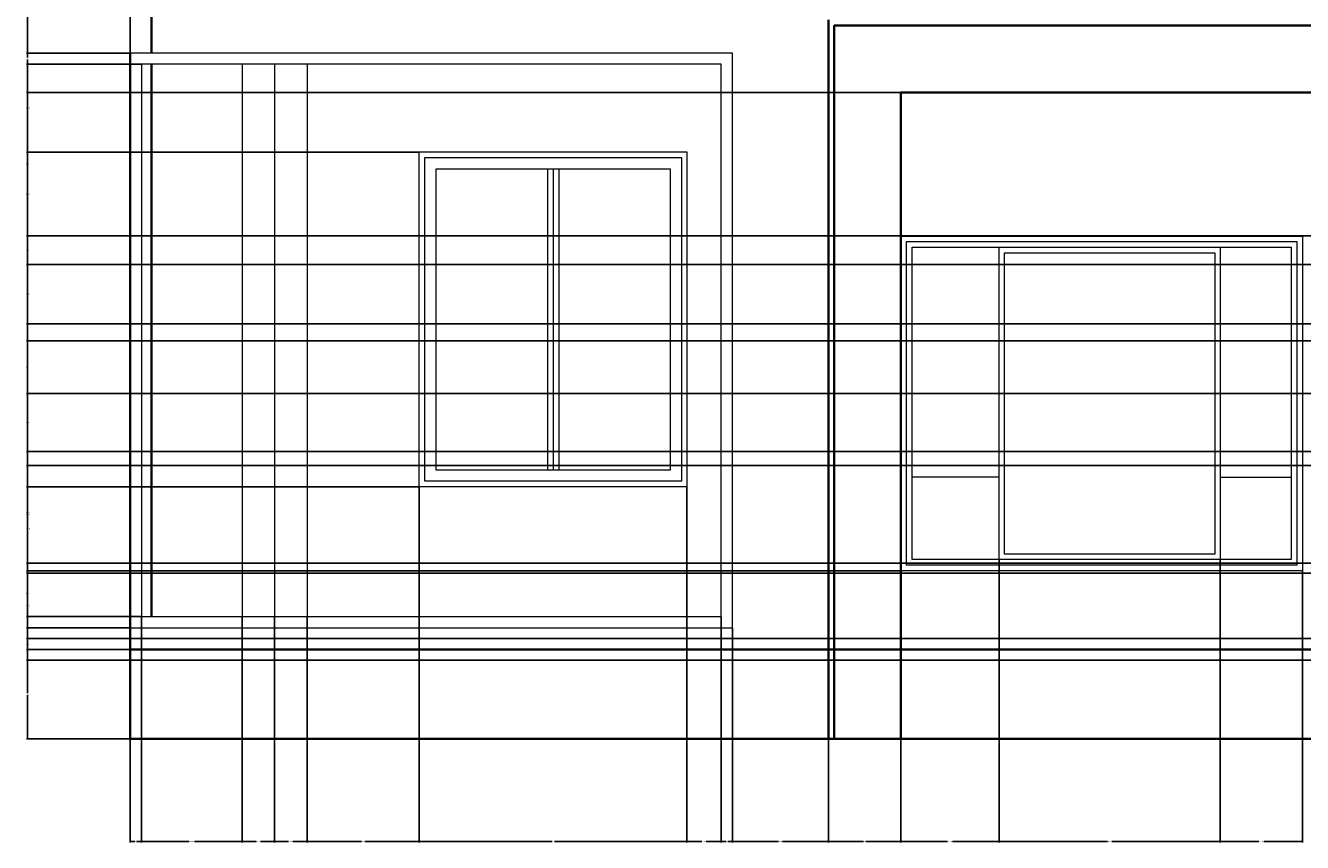
# Model space of a CAD drawing. Units: inches. Extents: x -7 to 391, y -12 to 303.
# Tile 1 of 5: x -7 to 222, y -12 to 134. Entities that reach past the tile are written whole.
import ezdxf

# ---------------------------------------------------------------- set-up
doc = ezdxf.new("R2010")
doc.units = ezdxf.units.IN
doc.header["$MEASUREMENT"] = 0
for name, color, linetype, lineweight in [('A-ANNO-DIMS', 2, 'Continuous', 18), ('A-DOOR', 3, 'Continuous', 18), ('A-ELEV', 7, 'Continuous', 35), ('A-GLAZ', 4, 'Continuous', 18)]:
    doc.layers.add(name, color=color, linetype=linetype, lineweight=lineweight)
doc.styles.get("Standard").update_dxf_attribs({"font": 'arial.ttf'})
doc.dimstyles.get("Standard").update_dxf_attribs({"dimtxt": 0.18, "dimasz": 0.18, "dimexe": 0.18, "dimexo": 0.0625, "dimgap": 0.09, "dimtad": 0, "dimtih": 1, "dimtoh": 1, "dimdec": 4, "dimzin": 0, "dimdsep": 46, "dimtxsty": 'Standard', "dimcen": 0.09, "dimadec": 0, "dimazin": 0, "dimtfac": 1, "dimtdec": 4, "dimtofl": 0, "dimtmove": 0, "dimatfit": 3, "dimfxl": 1, "dimtolj": 1, "dimtzin": 0, "dimarcsym": 0})

# ---------------------------------------------------------------- blocks, each defined once
blk = doc.blocks.new('*D1')
at = {"layer": 'A-ANNO-DIMS', "color": 0, "lineweight": -2, "transparency": 16777216}
for p, q in [((372.08, 122.18), (390.6, 122.18)), ((390.42, 122), (390.42, 64.44)), ((390.42, 6.53), (390.42, 64.08)), ((150.31, 6.35), (390.6, 6.35))]:
    blk.add_line(p, q, dxfattribs=at)
at = {"layer": 'A-ANNO-DIMS', "color": 0, "transparency": 16777216}
for points in [[(390.39, 122), (390.45, 122), (390.42, 122.18)], [(390.39, 6.53), (390.45, 6.53), (390.42, 6.35)]]:
    blk.add_solid(points, dxfattribs=at)
at = {"layer": 'Defpoints', "color": 0, "transparency": 16777216}
for p in [(372.02, 122.18), (390.42, 122.18), (150.24, 6.35)]:
    blk.add_point(p, dxfattribs=at)
at = {"layer": 'A-ANNO-DIMS', "color": 0, "transparency": 16777216, "insert": (390.42, 64.26), "char_height": 0.18, "attachment_point": 5}
blk.add_mtext('\\A1;115.83', dxfattribs=at)
blk = doc.blocks.new('*D7')
at = {"layer": 'A-ANNO-DIMS', "color": 0, "lineweight": -2, "transparency": 16777216}
for p, q in [((11.96, 22.35), (-6.56, 22.35)), ((-6.38, 22.17), (-6.38, 14.53)), ((-6.38, 6.53), (-6.38, 14.16)), ((11.96, 6.35), (-6.56, 6.35))]:
    blk.add_line(p, q, dxfattribs=at)
at = {"layer": 'A-ANNO-DIMS', "color": 0, "transparency": 16777216}
for points in [[(-6.41, 22.17), (-6.35, 22.17), (-6.38, 22.35)], [(-6.41, 6.53), (-6.35, 6.53), (-6.38, 6.35)]]:
    blk.add_solid(points, dxfattribs=at)
at = {"layer": 'Defpoints', "color": 0, "transparency": 16777216}
for p in [(-6.38, 22.35), (12.02, 22.35), (12.02, 6.35)]:
    blk.add_point(p, dxfattribs=at)
at = {"layer": 'A-ANNO-DIMS', "color": 0, "transparency": 16777216, "insert": (-6.38, 14.35), "char_height": 0.18, "attachment_point": 5}
blk.add_mtext('\\A1;16', dxfattribs=at)
blk = doc.blocks.new('*D8')
at = {"layer": 'A-ANNO-DIMS', "color": 0, "lineweight": -2, "transparency": 16777216}
for p, q in [((11.96, 26.25), (-6.56, 26.25)), ((-6.38, 26.07), (-6.38, 24.48)), ((-6.38, 22.53), (-6.38, 24.12)), ((11.96, 22.35), (-6.56, 22.35))]:
    blk.add_line(p, q, dxfattribs=at)
at = {"layer": 'A-ANNO-DIMS', "color": 0, "transparency": 16777216}
for points in [[(-6.41, 26.07), (-6.35, 26.07), (-6.38, 26.25)], [(-6.41, 22.53), (-6.35, 22.53), (-6.38, 22.35)]]:
    blk.add_solid(points, dxfattribs=at)
at = {"layer": 'Defpoints', "color": 0, "transparency": 16777216}
for p in [(-6.38, 26.25), (12.02, 26.25), (12.02, 22.35)]:
    blk.add_point(p, dxfattribs=at)
at = {"layer": 'A-ANNO-DIMS', "color": 0, "transparency": 16777216, "insert": (-6.38, 24.3), "char_height": 0.18, "attachment_point": 5}
blk.add_mtext('\\A1;3.905', dxfattribs=at)
blk = doc.blocks.new('*D9')
at = {"layer": 'A-ANNO-DIMS', "color": 0, "lineweight": -2, "transparency": 16777216}
for p, q in [((13.96, 28.25), (-6.56, 28.25)), ((-6.38, 28.07), (-6.38, 27.43)), ((11.96, 26.25), (-6.56, 26.25)), ((-6.38, 26.43), (-6.38, 27.07))]:
    blk.add_line(p, q, dxfattribs=at)
at = {"layer": 'A-ANNO-DIMS', "color": 0, "transparency": 16777216}
for points in [[(-6.41, 28.07), (-6.35, 28.07), (-6.38, 28.25)], [(-6.41, 26.43), (-6.35, 26.43), (-6.38, 26.25)]]:
    blk.add_solid(points, dxfattribs=at)
at = {"layer": 'Defpoints', "color": 0, "transparency": 16777216}
for p in [(-6.38, 28.25), (14.02, 28.25), (12.02, 26.25)]:
    blk.add_point(p, dxfattribs=at)
at = {"layer": 'A-ANNO-DIMS', "color": 0, "transparency": 16777216, "insert": (-6.38, 27.25), "char_height": 0.18, "attachment_point": 5}
blk.add_mtext('\\A1;2', dxfattribs=at)
blk = doc.blocks.new('*D10')
at = {"layer": 'A-ANNO-DIMS', "color": 0, "lineweight": -2, "transparency": 16777216}
for p, q in [((150.18, 36.46), (-6.56, 36.46)), ((-6.38, 36.28), (-6.38, 32.54)), ((-6.38, 28.43), (-6.38, 32.17)), ((13.96, 28.25), (-6.56, 28.25))]:
    blk.add_line(p, q, dxfattribs=at)
at = {"layer": 'A-ANNO-DIMS', "color": 0, "transparency": 16777216}
for points in [[(-6.41, 36.28), (-6.35, 36.28), (-6.38, 36.46)], [(-6.41, 28.43), (-6.35, 28.43), (-6.38, 28.25)]]:
    blk.add_solid(points, dxfattribs=at)
at = {"layer": 'Defpoints', "color": 0, "transparency": 16777216}
for p in [(-6.38, 36.46), (150.24, 36.46), (14.02, 28.25)]:
    blk.add_point(p, dxfattribs=at)
at = {"layer": 'A-ANNO-DIMS', "color": 0, "transparency": 16777216, "insert": (-6.38, 32.35), "char_height": 0.18, "attachment_point": 5}
blk.add_mtext('\\A1;8.206', dxfattribs=at)
blk = doc.blocks.new('*D11')
at = {"layer": 'A-ANNO-DIMS', "color": 0, "lineweight": -2, "transparency": 16777216}
for p, q in [((63.8, 51.51), (-6.56, 51.51)), ((-6.38, 51.33), (-6.38, 44.17)), ((-6.38, 36.64), (-6.38, 43.8)), ((150.18, 36.46), (-6.56, 36.46))]:
    blk.add_line(p, q, dxfattribs=at)
at = {"layer": 'A-ANNO-DIMS', "color": 0, "transparency": 16777216}
for points in [[(-6.41, 51.33), (-6.35, 51.33), (-6.38, 51.51)], [(-6.41, 36.64), (-6.35, 36.64), (-6.38, 36.46)]]:
    blk.add_solid(points, dxfattribs=at)
at = {"layer": 'Defpoints', "color": 0, "transparency": 16777216}
for p in [(-6.38, 51.51), (63.86, 51.51), (150.24, 36.46)]:
    blk.add_point(p, dxfattribs=at)
at = {"layer": 'A-ANNO-DIMS', "color": 0, "transparency": 16777216, "insert": (-6.38, 43.98), "char_height": 0.18, "attachment_point": 5}
blk.add_mtext('\\A1;15.058', dxfattribs=at)
blk = doc.blocks.new('*D12')
at = {"layer": 'A-ANNO-DIMS', "color": 0, "lineweight": -2, "transparency": 16777216}
for p, q in [((150.18, 96.46), (-6.56, 96.46)), ((-6.38, 96.28), (-6.38, 74.17)), ((-6.38, 51.69), (-6.38, 73.8)), ((63.8, 51.51), (-6.56, 51.51))]:
    blk.add_line(p, q, dxfattribs=at)
at = {"layer": 'A-ANNO-DIMS', "color": 0, "transparency": 16777216}
for points in [[(-6.41, 96.28), (-6.35, 96.28), (-6.38, 96.46)], [(-6.41, 51.69), (-6.35, 51.69), (-6.38, 51.51)]]:
    blk.add_solid(points, dxfattribs=at)
at = {"layer": 'Defpoints', "color": 0, "transparency": 16777216}
for p in [(-6.38, 96.46), (150.24, 96.46), (63.86, 51.51)]:
    blk.add_point(p, dxfattribs=at)
at = {"layer": 'A-ANNO-DIMS', "color": 0, "transparency": 16777216, "insert": (-6.38, 73.98), "char_height": 0.18, "attachment_point": 5}
blk.add_mtext('\\A1;44.94', dxfattribs=at)
blk = doc.blocks.new('*D13')
at = {"layer": 'A-ANNO-DIMS', "color": 0, "lineweight": -2, "transparency": 16777216}
for p, q in [((63.8, 111.51), (-6.56, 111.51)), ((-6.38, 111.33), (-6.38, 104.17)), ((-6.38, 96.64), (-6.38, 103.8)), ((150.18, 96.46), (-6.56, 96.46))]:
    blk.add_line(p, q, dxfattribs=at)
at = {"layer": 'A-ANNO-DIMS', "color": 0, "transparency": 16777216}
for points in [[(-6.41, 111.33), (-6.35, 111.33), (-6.38, 111.51)], [(-6.41, 96.64), (-6.35, 96.64), (-6.38, 96.46)]]:
    blk.add_solid(points, dxfattribs=at)
at = {"layer": 'Defpoints', "color": 0, "transparency": 16777216}
for p in [(-6.38, 111.51), (63.86, 111.51), (150.24, 96.46)]:
    blk.add_point(p, dxfattribs=at)
at = {"layer": 'A-ANNO-DIMS', "color": 0, "transparency": 16777216, "insert": (-6.38, 103.98), "char_height": 0.18, "attachment_point": 5}
blk.add_mtext('\\A1;15.058', dxfattribs=at)
blk = doc.blocks.new('*D14')
at = {"layer": 'A-ANNO-DIMS', "color": 0, "lineweight": -2, "transparency": 16777216}
for p, q in [((13.96, 127.25), (-6.56, 127.25)), ((-6.38, 127.07), (-6.38, 119.56)), ((-6.38, 111.69), (-6.38, 119.2)), ((63.8, 111.51), (-6.56, 111.51))]:
    blk.add_line(p, q, dxfattribs=at)
at = {"layer": 'A-ANNO-DIMS', "color": 0, "transparency": 16777216}
for points in [[(-6.41, 127.07), (-6.35, 127.07), (-6.38, 127.25)], [(-6.41, 111.69), (-6.35, 111.69), (-6.38, 111.51)]]:
    blk.add_solid(points, dxfattribs=at)
at = {"layer": 'Defpoints', "color": 0, "transparency": 16777216}
for p in [(-6.38, 127.25), (14.02, 127.25), (63.86, 111.51)]:
    blk.add_point(p, dxfattribs=at)
at = {"layer": 'A-ANNO-DIMS', "color": 0, "transparency": 16777216, "insert": (-6.38, 119.38), "char_height": 0.18, "attachment_point": 5}
blk.add_mtext('\\A1;15.736', dxfattribs=at)
blk = doc.blocks.new('*D15')
at = {"layer": 'A-ANNO-DIMS', "color": 0, "lineweight": -2, "transparency": 16777216}
for p, q in [((11.96, 129.25), (-6.56, 129.25)), ((-6.38, 129.07), (-6.38, 128.43)), ((13.96, 127.25), (-6.56, 127.25)), ((-6.38, 127.43), (-6.38, 128.07))]:
    blk.add_line(p, q, dxfattribs=at)
at = {"layer": 'A-ANNO-DIMS', "color": 0, "transparency": 16777216}
for points in [[(-6.41, 129.07), (-6.35, 129.07), (-6.38, 129.25)], [(-6.41, 127.43), (-6.35, 127.43), (-6.38, 127.25)]]:
    blk.add_solid(points, dxfattribs=at)
at = {"layer": 'Defpoints', "color": 0, "transparency": 16777216}
for p in [(-6.38, 129.25), (12.02, 129.25), (14.02, 127.25)]:
    blk.add_point(p, dxfattribs=at)
at = {"layer": 'A-ANNO-DIMS', "color": 0, "transparency": 16777216, "insert": (-6.38, 128.25), "char_height": 0.18, "attachment_point": 5}
blk.add_mtext('\\A1;2', dxfattribs=at)
blk = doc.blocks.new('*D16')
at = {"layer": 'A-ANNO-DIMS', "color": 0, "lineweight": -2, "transparency": 16777216}
for p, q in [((15.76, 154.35), (-6.56, 154.35)), ((-6.38, 154.17), (-6.38, 141.98)), ((-6.38, 129.43), (-6.38, 141.62)), ((11.96, 129.25), (-6.56, 129.25))]:
    blk.add_line(p, q, dxfattribs=at)
at = {"layer": 'A-ANNO-DIMS', "color": 0, "transparency": 16777216}
for points in [[(-6.41, 154.17), (-6.35, 154.17), (-6.38, 154.35)], [(-6.41, 129.43), (-6.35, 129.43), (-6.38, 129.25)]]:
    blk.add_solid(points, dxfattribs=at)
at = {"layer": 'Defpoints', "color": 0, "transparency": 16777216}
for p in [(-6.38, 154.35), (15.82, 154.35), (12.02, 129.25)]:
    blk.add_point(p, dxfattribs=at)
at = {"layer": 'A-ANNO-DIMS', "color": 0, "transparency": 16777216, "insert": (-6.38, 141.8), "char_height": 0.18, "attachment_point": 5}
blk.add_mtext('\\A1;25.095', dxfattribs=at)
blk = doc.blocks.new('*D17')
at = {"layer": 'A-ANNO-DIMS', "color": 0, "lineweight": -2, "transparency": 16777216}
for p, q in [((150.18, 122.18), (-6.56, 122.18)), ((-6.38, 122), (-6.38, 109.5)), ((-6.38, 96.64), (-6.38, 109.13)), ((150.18, 96.46), (-6.56, 96.46))]:
    blk.add_line(p, q, dxfattribs=at)
at = {"layer": 'A-ANNO-DIMS', "color": 0, "transparency": 16777216}
for points in [[(-6.41, 122), (-6.35, 122), (-6.38, 122.18)], [(-6.41, 96.64), (-6.35, 96.64), (-6.38, 96.46)]]:
    blk.add_solid(points, dxfattribs=at)
at = {"layer": 'Defpoints', "color": 0, "transparency": 16777216}
for p in [(-6.38, 122.18), (150.24, 122.18), (150.24, 96.46)]:
    blk.add_point(p, dxfattribs=at)
at = {"layer": 'A-ANNO-DIMS', "color": 0, "transparency": 16777216, "insert": (-6.38, 109.32), "char_height": 0.18, "attachment_point": 5}
blk.add_mtext('\\A1;25.72', dxfattribs=at)
blk = doc.blocks.new('*D18')
at = {"layer": 'A-ANNO-DIMS', "color": 0, "lineweight": -2, "transparency": 16777216}
for p, q in [((12.02, 129.31), (12.02, 303.01)), ((12.2, 302.83), (13.53, 302.83)), ((15.64, 302.83), (14.31, 302.83)), ((15.82, 154.41), (15.82, 303.01))]:
    blk.add_line(p, q, dxfattribs=at)
at = {"layer": 'A-ANNO-DIMS', "color": 0, "transparency": 16777216}
for points in [[(12.2, 302.86), (12.2, 302.8), (12.02, 302.83)], [(15.64, 302.86), (15.64, 302.8), (15.82, 302.83)]]:
    blk.add_solid(points, dxfattribs=at)
at = {"layer": 'Defpoints', "color": 0, "transparency": 16777216}
for p in [(15.82, 302.83), (15.82, 154.35), (12.02, 129.25)]:
    blk.add_point(p, dxfattribs=at)
at = {"layer": 'A-ANNO-DIMS', "color": 0, "transparency": 16777216, "insert": (13.92, 302.83), "char_height": 0.18, "attachment_point": 5}
blk.add_mtext('\\A1;3.799', dxfattribs=at)
blk = doc.blocks.new('*D25')
at = {"layer": 'A-ANNO-DIMS', "color": 0, "lineweight": -2, "transparency": 16777216}
for p, q in [((14.02, 28.19), (14.02, -12.23)), ((12.02, 6.28), (12.02, -12.23)), ((12.2, -12.05), (12.87, -12.05)), ((13.84, -12.05), (13.17, -12.05))]:
    blk.add_line(p, q, dxfattribs=at)
at = {"layer": 'A-ANNO-DIMS', "color": 0, "transparency": 16777216}
for points in [[(12.2, -12.02), (12.2, -12.08), (12.02, -12.05)], [(13.84, -12.02), (13.84, -12.08), (14.02, -12.05)]]:
    blk.add_solid(points, dxfattribs=at)
at = {"layer": 'Defpoints', "color": 0, "transparency": 16777216}
for p in [(14.02, 28.25), (12.02, 6.35), (14.02, -12.05)]:
    blk.add_point(p, dxfattribs=at)
at = {"layer": 'A-ANNO-DIMS', "color": 0, "transparency": 16777216, "insert": (13.02, -12.05), "char_height": 0.18, "attachment_point": 5}
blk.add_mtext('\\A1;2', dxfattribs=at)
blk = doc.blocks.new('*D26')
at = {"layer": 'A-ANNO-DIMS', "color": 0, "lineweight": -2, "transparency": 16777216}
for p, q in [((14.02, 28.19), (14.02, -12.23)), ((32.11, 28.19), (32.11, -12.23)), ((14.2, -12.05), (22.61, -12.05)), ((31.93, -12.05), (23.52, -12.05))]:
    blk.add_line(p, q, dxfattribs=at)
at = {"layer": 'A-ANNO-DIMS', "color": 0, "transparency": 16777216}
for points in [[(14.2, -12.02), (14.2, -12.08), (14.02, -12.05)], [(31.93, -12.02), (31.93, -12.08), (32.11, -12.05)]]:
    blk.add_solid(points, dxfattribs=at)
at = {"layer": 'Defpoints', "color": 0, "transparency": 16777216}
for p in [(14.02, 28.25), (32.11, 28.25), (32.11, -12.05)]:
    blk.add_point(p, dxfattribs=at)
at = {"layer": 'A-ANNO-DIMS', "color": 0, "transparency": 16777216, "insert": (23.07, -12.05), "char_height": 0.18, "attachment_point": 5}
blk.add_mtext('\\A1;18.092', dxfattribs=at)
blk = doc.blocks.new('*D27')
at = {"layer": 'A-ANNO-DIMS', "color": 0, "lineweight": -2, "transparency": 16777216}
for p, q in [((32.11, 28.19), (32.11, -12.23)), ((37.87, 28.19), (37.87, -12.23)), ((32.29, -12.05), (34.6, -12.05)), ((37.69, -12.05), (35.39, -12.05))]:
    blk.add_line(p, q, dxfattribs=at)
at = {"layer": 'A-ANNO-DIMS', "color": 0, "transparency": 16777216}
for points in [[(32.29, -12.02), (32.29, -12.08), (32.11, -12.05)], [(37.69, -12.02), (37.69, -12.08), (37.87, -12.05)]]:
    blk.add_solid(points, dxfattribs=at)
at = {"layer": 'Defpoints', "color": 0, "transparency": 16777216}
for p in [(32.11, 28.25), (37.87, 28.25), (37.87, -12.05)]:
    blk.add_point(p, dxfattribs=at)
at = {"layer": 'A-ANNO-DIMS', "color": 0, "transparency": 16777216, "insert": (34.99, -12.05), "char_height": 0.18, "attachment_point": 5}
blk.add_mtext('\\A1;5.757', dxfattribs=at)
blk = doc.blocks.new('*D28')
at = {"layer": 'A-ANNO-DIMS', "color": 0, "lineweight": -2, "transparency": 16777216}
for p, q in [((37.87, 28.19), (37.87, -12.23)), ((43.76, 28.19), (43.76, -12.23)), ((38.05, -12.05), (40.42, -12.05)), ((43.58, -12.05), (41.21, -12.05))]:
    blk.add_line(p, q, dxfattribs=at)
at = {"layer": 'A-ANNO-DIMS', "color": 0, "transparency": 16777216}
for points in [[(38.05, -12.02), (38.05, -12.08), (37.87, -12.05)], [(43.58, -12.02), (43.58, -12.08), (43.76, -12.05)]]:
    blk.add_solid(points, dxfattribs=at)
at = {"layer": 'Defpoints', "color": 0, "transparency": 16777216}
for p in [(37.87, 28.25), (43.76, 28.25), (43.76, -12.05)]:
    blk.add_point(p, dxfattribs=at)
at = {"layer": 'A-ANNO-DIMS', "color": 0, "transparency": 16777216, "insert": (40.81, -12.05), "char_height": 0.18, "attachment_point": 5}
blk.add_mtext('\\A1;5.887', dxfattribs=at)
blk = doc.blocks.new('*D29')
at = {"layer": 'A-ANNO-DIMS', "color": 0, "lineweight": -2, "transparency": 16777216}
for p, q in [((63.86, 51.45), (63.86, -12.23)), ((43.76, 28.19), (43.76, -12.23)), ((43.94, -12.05), (53.5, -12.05)), ((63.68, -12.05), (54.12, -12.05))]:
    blk.add_line(p, q, dxfattribs=at)
at = {"layer": 'A-ANNO-DIMS', "color": 0, "transparency": 16777216}
for points in [[(43.94, -12.02), (43.94, -12.08), (43.76, -12.05)], [(63.68, -12.02), (63.68, -12.08), (63.86, -12.05)]]:
    blk.add_solid(points, dxfattribs=at)
at = {"layer": 'Defpoints', "color": 0, "transparency": 16777216}
for p in [(63.86, 51.51), (43.76, 28.25), (63.86, -12.05)]:
    blk.add_point(p, dxfattribs=at)
at = {"layer": 'A-ANNO-DIMS', "color": 0, "transparency": 16777216, "insert": (53.81, -12.05), "char_height": 0.18, "attachment_point": 5}
blk.add_mtext('\\A1;20.1', dxfattribs=at)
blk = doc.blocks.new('*D30')
at = {"layer": 'A-ANNO-DIMS', "color": 0, "lineweight": -2, "transparency": 16777216}
for p, q in [((63.86, 51.45), (63.86, -12.23)), ((111.86, 51.45), (111.86, -12.23)), ((64.04, -12.05), (87.64, -12.05)), ((111.68, -12.05), (88.08, -12.05))]:
    blk.add_line(p, q, dxfattribs=at)
at = {"layer": 'A-ANNO-DIMS', "color": 0, "transparency": 16777216}
for points in [[(64.04, -12.02), (64.04, -12.08), (63.86, -12.05)], [(111.68, -12.02), (111.68, -12.08), (111.86, -12.05)]]:
    blk.add_solid(points, dxfattribs=at)
at = {"layer": 'Defpoints', "color": 0, "transparency": 16777216}
for p in [(63.86, 51.51), (111.86, 51.51), (111.86, -12.05)]:
    blk.add_point(p, dxfattribs=at)
at = {"layer": 'A-ANNO-DIMS', "color": 0, "transparency": 16777216, "insert": (87.86, -12.05), "char_height": 0.18, "attachment_point": 5}
blk.add_mtext('\\A1;48', dxfattribs=at)
blk = doc.blocks.new('*D31')
at = {"layer": 'A-ANNO-DIMS', "color": 0, "lineweight": -2, "transparency": 16777216}
for p, q in [((111.86, 51.45), (111.86, -12.23)), ((118.02, 28.19), (118.02, -12.23)), ((112.04, -12.05), (114.55, -12.05)), ((117.84, -12.05), (115.33, -12.05))]:
    blk.add_line(p, q, dxfattribs=at)
at = {"layer": 'A-ANNO-DIMS', "color": 0, "transparency": 16777216}
for points in [[(112.04, -12.02), (112.04, -12.08), (111.86, -12.05)], [(117.84, -12.02), (117.84, -12.08), (118.02, -12.05)]]:
    blk.add_solid(points, dxfattribs=at)
at = {"layer": 'Defpoints', "color": 0, "transparency": 16777216}
for p in [(111.86, 51.51), (118.02, 28.25), (118.02, -12.05)]:
    blk.add_point(p, dxfattribs=at)
at = {"layer": 'A-ANNO-DIMS', "color": 0, "transparency": 16777216, "insert": (114.94, -12.05), "char_height": 0.18, "attachment_point": 5}
blk.add_mtext('\\A1;6.163', dxfattribs=at)
blk = doc.blocks.new('*D32')
at = {"layer": 'A-ANNO-DIMS', "color": 0, "lineweight": -2, "transparency": 16777216}
for p, q in [((118.02, 28.19), (118.02, -12.23)), ((120.02, 26.19), (120.02, -12.23)), ((118.2, -12.05), (118.87, -12.05)), ((119.84, -12.05), (119.17, -12.05))]:
    blk.add_line(p, q, dxfattribs=at)
at = {"layer": 'A-ANNO-DIMS', "color": 0, "transparency": 16777216}
for points in [[(118.2, -12.02), (118.2, -12.08), (118.02, -12.05)], [(119.84, -12.02), (119.84, -12.08), (120.02, -12.05)]]:
    blk.add_solid(points, dxfattribs=at)
at = {"layer": 'Defpoints', "color": 0, "transparency": 16777216}
for p in [(118.02, 28.25), (120.02, 26.25), (120.02, -12.05)]:
    blk.add_point(p, dxfattribs=at)
at = {"layer": 'A-ANNO-DIMS', "color": 0, "transparency": 16777216, "insert": (119.02, -12.05), "char_height": 0.18, "attachment_point": 5}
blk.add_mtext('\\A1;2', dxfattribs=at)
blk = doc.blocks.new('*D33')
at = {"layer": 'A-ANNO-DIMS', "color": 0, "lineweight": -2, "transparency": 16777216}
for p, q in [((120.02, 26.19), (120.02, -12.23)), ((137.24, 6.28), (137.24, -12.23)), ((120.2, -12.05), (128.25, -12.05)), ((137.06, -12.05), (129.02, -12.05))]:
    blk.add_line(p, q, dxfattribs=at)
at = {"layer": 'A-ANNO-DIMS', "color": 0, "transparency": 16777216}
for points in [[(120.2, -12.02), (120.2, -12.08), (120.02, -12.05)], [(137.06, -12.02), (137.06, -12.08), (137.24, -12.05)]]:
    blk.add_solid(points, dxfattribs=at)
at = {"layer": 'Defpoints', "color": 0, "transparency": 16777216}
for p in [(120.02, 26.25), (137.24, 6.35), (137.24, -12.05)]:
    blk.add_point(p, dxfattribs=at)
at = {"layer": 'A-ANNO-DIMS', "color": 0, "transparency": 16777216, "insert": (128.63, -12.05), "char_height": 0.18, "attachment_point": 5}
blk.add_mtext('\\A1;17.22', dxfattribs=at)
blk = doc.blocks.new('*D34')
at = {"layer": 'A-ANNO-DIMS', "color": 0, "lineweight": -2, "transparency": 16777216}
for p, q in [((137.24, 6.28), (137.24, -12.23)), ((150.24, 6.28), (150.24, -12.23)), ((137.42, -12.05), (143.53, -12.05)), ((150.06, -12.05), (143.95, -12.05))]:
    blk.add_line(p, q, dxfattribs=at)
at = {"layer": 'A-ANNO-DIMS', "color": 0, "transparency": 16777216}
for points in [[(137.42, -12.02), (137.42, -12.08), (137.24, -12.05)], [(150.06, -12.02), (150.06, -12.08), (150.24, -12.05)]]:
    blk.add_solid(points, dxfattribs=at)
at = {"layer": 'Defpoints', "color": 0, "transparency": 16777216}
for p in [(137.24, 6.35), (150.24, 6.35), (150.24, -12.05)]:
    blk.add_point(p, dxfattribs=at)
at = {"layer": 'A-ANNO-DIMS', "color": 0, "transparency": 16777216, "insert": (143.74, -12.05), "char_height": 0.18, "attachment_point": 5}
blk.add_mtext('\\A1;13', dxfattribs=at)
blk = doc.blocks.new('*D35')
at = {"layer": 'A-ANNO-DIMS', "color": 0, "lineweight": -2, "transparency": 16777216}
for p, q in [((167.84, 38.39), (167.84, -12.23)), ((150.24, 36.39), (150.24, -12.23)), ((150.42, -12.05), (158.58, -12.05)), ((167.66, -12.05), (159.49, -12.05))]:
    blk.add_line(p, q, dxfattribs=at)
at = {"layer": 'A-ANNO-DIMS', "color": 0, "transparency": 16777216}
for points in [[(150.42, -12.02), (150.42, -12.08), (150.24, -12.05)], [(167.66, -12.02), (167.66, -12.08), (167.84, -12.05)]]:
    blk.add_solid(points, dxfattribs=at)
at = {"layer": 'Defpoints', "color": 0, "transparency": 16777216}
for p in [(167.84, 38.46), (150.24, 36.46), (167.84, -12.05)]:
    blk.add_point(p, dxfattribs=at)
at = {"layer": 'A-ANNO-DIMS', "color": 0, "transparency": 16777216, "insert": (159.04, -12.05), "char_height": 0.18, "attachment_point": 5}
blk.add_mtext('\\A1;17.593', dxfattribs=at)
blk = doc.blocks.new('*D36')
at = {"layer": 'A-ANNO-DIMS', "color": 0, "lineweight": -2, "transparency": 16777216}
for p, q in [((167.84, 38.39), (167.84, -12.23)), ((207.51, 38.39), (207.51, -12.23)), ((168.02, -12.05), (187.28, -12.05)), ((207.33, -12.05), (188.07, -12.05))]:
    blk.add_line(p, q, dxfattribs=at)
at = {"layer": 'A-ANNO-DIMS', "color": 0, "transparency": 16777216}
for points in [[(168.02, -12.02), (168.02, -12.08), (167.84, -12.05)], [(207.33, -12.02), (207.33, -12.08), (207.51, -12.05)]]:
    blk.add_solid(points, dxfattribs=at)
at = {"layer": 'Defpoints', "color": 0, "transparency": 16777216}
for p in [(167.84, 38.46), (207.51, 38.46), (207.51, -12.05)]:
    blk.add_point(p, dxfattribs=at)
at = {"layer": 'A-ANNO-DIMS', "color": 0, "transparency": 16777216, "insert": (187.67, -12.05), "char_height": 0.18, "attachment_point": 5}
blk.add_mtext('\\A1;39.67', dxfattribs=at)
blk = doc.blocks.new('*D37')
at = {"layer": 'A-ANNO-DIMS', "color": 0, "lineweight": -2, "transparency": 16777216}
for p, q in [((207.51, 38.39), (207.51, -12.23)), ((222.24, 36.39), (222.24, -12.23)), ((207.69, -12.05), (214.42, -12.05)), ((222.06, -12.05), (215.33, -12.05))]:
    blk.add_line(p, q, dxfattribs=at)
at = {"layer": 'A-ANNO-DIMS', "color": 0, "transparency": 16777216}
for points in [[(207.69, -12.02), (207.69, -12.08), (207.51, -12.05)], [(222.06, -12.02), (222.06, -12.08), (222.24, -12.05)]]:
    blk.add_solid(points, dxfattribs=at)
at = {"layer": 'Defpoints', "color": 0, "transparency": 16777216}
for p in [(207.51, 38.46), (222.24, 36.46), (222.24, -12.05)]:
    blk.add_point(p, dxfattribs=at)
at = {"layer": 'A-ANNO-DIMS', "color": 0, "transparency": 16777216, "insert": (214.88, -12.05), "char_height": 0.18, "attachment_point": 5}
blk.add_mtext('\\A1;14.734', dxfattribs=at)
blk = doc.blocks.new('*D64')
at = {"layer": 'A-ANNO-DIMS', "color": 0, "lineweight": -2, "transparency": 16777216}
for p, q in [((264.07, 24.3), (-6.56, 24.3)), ((-6.38, 24.12), (-6.38, 23.5)), ((-6.38, 22.53), (-6.38, 23.14)), ((246.68, 22.35), (-6.56, 22.35))]:
    blk.add_line(p, q, dxfattribs=at)
at = {"layer": 'A-ANNO-DIMS', "color": 0, "transparency": 16777216}
for points in [[(-6.41, 24.12), (-6.35, 24.12), (-6.38, 24.3)], [(-6.41, 22.53), (-6.35, 22.53), (-6.38, 22.35)]]:
    blk.add_solid(points, dxfattribs=at)
at = {"layer": 'Defpoints', "color": 0, "transparency": 16777216}
for p in [(-6.38, 24.3), (264.13, 24.3), (246.74, 22.35)]:
    blk.add_point(p, dxfattribs=at)
at = {"layer": 'A-ANNO-DIMS', "color": 0, "transparency": 16777216, "insert": (-6.38, 23.32), "char_height": 0.18, "attachment_point": 5}
blk.add_mtext('\\A1;1.952', dxfattribs=at)
blk = doc.blocks.new('*D65')
at = {"layer": 'A-ANNO-DIMS', "color": 0, "lineweight": -2, "transparency": 16777216}
for p, q in [((264.07, 36.01), (-6.56, 36.01)), ((-6.38, 35.83), (-6.38, 30.34)), ((-6.38, 24.48), (-6.38, 29.97)), ((264.07, 24.3), (-6.56, 24.3))]:
    blk.add_line(p, q, dxfattribs=at)
at = {"layer": 'A-ANNO-DIMS', "color": 0, "transparency": 16777216}
for points in [[(-6.41, 35.83), (-6.35, 35.83), (-6.38, 36.01)], [(-6.41, 24.48), (-6.35, 24.48), (-6.38, 24.3)]]:
    blk.add_solid(points, dxfattribs=at)
at = {"layer": 'Defpoints', "color": 0, "transparency": 16777216}
for p in [(-6.38, 36.01), (264.13, 36.01), (264.13, 24.3)]:
    blk.add_point(p, dxfattribs=at)
at = {"layer": 'A-ANNO-DIMS', "color": 0, "transparency": 16777216, "insert": (-6.38, 30.16), "char_height": 0.18, "attachment_point": 5}
blk.add_mtext('\\A1;11.716', dxfattribs=at)
blk = doc.blocks.new('*D66')
at = {"layer": 'A-ANNO-DIMS', "color": 0, "lineweight": -2, "transparency": 16777216}
for p, q in [((264.07, 57.83), (-6.56, 57.83)), ((-6.38, 57.65), (-6.38, 47.1)), ((-6.38, 36.19), (-6.38, 46.74)), ((264.07, 36.01), (-6.56, 36.01))]:
    blk.add_line(p, q, dxfattribs=at)
at = {"layer": 'A-ANNO-DIMS', "color": 0, "transparency": 16777216}
for points in [[(-6.41, 57.65), (-6.35, 57.65), (-6.38, 57.83)], [(-6.41, 36.19), (-6.35, 36.19), (-6.38, 36.01)]]:
    blk.add_solid(points, dxfattribs=at)
at = {"layer": 'Defpoints', "color": 0, "transparency": 16777216}
for p in [(-6.38, 57.83), (264.13, 57.83), (264.13, 36.01)]:
    blk.add_point(p, dxfattribs=at)
at = {"layer": 'A-ANNO-DIMS', "color": 0, "transparency": 16777216, "insert": (-6.38, 46.92), "char_height": 0.18, "attachment_point": 5}
blk.add_mtext('\\A1;21.82', dxfattribs=at)
blk = doc.blocks.new('*D67')
at = {"layer": 'A-ANNO-DIMS', "color": 0, "lineweight": -2, "transparency": 16777216}
for p, q in [((264.07, 68.22), (-6.56, 68.22)), ((-6.38, 68.04), (-6.38, 63.21)), ((-6.38, 58.01), (-6.38, 62.84)), ((264.07, 57.83), (-6.56, 57.83))]:
    blk.add_line(p, q, dxfattribs=at)
at = {"layer": 'A-ANNO-DIMS', "color": 0, "transparency": 16777216}
for points in [[(-6.41, 68.04), (-6.35, 68.04), (-6.38, 68.22)], [(-6.41, 58.01), (-6.35, 58.01), (-6.38, 57.83)]]:
    blk.add_solid(points, dxfattribs=at)
at = {"layer": 'Defpoints', "color": 0, "transparency": 16777216}
for p in [(-6.38, 68.22), (264.13, 68.22), (264.13, 57.83)]:
    blk.add_point(p, dxfattribs=at)
at = {"layer": 'A-ANNO-DIMS', "color": 0, "transparency": 16777216, "insert": (-6.38, 63.03), "char_height": 0.18, "attachment_point": 5}
blk.add_mtext('\\A1;10.388', dxfattribs=at)
blk = doc.blocks.new('*D68')
at = {"layer": 'A-ANNO-DIMS', "color": 0, "lineweight": -2, "transparency": 16777216}
for p, q in [((264.07, 77.69), (-6.56, 77.69)), ((-6.38, 77.51), (-6.38, 73.14)), ((-6.38, 68.4), (-6.38, 72.77)), ((264.07, 68.22), (-6.56, 68.22))]:
    blk.add_line(p, q, dxfattribs=at)
at = {"layer": 'A-ANNO-DIMS', "color": 0, "transparency": 16777216}
for points in [[(-6.41, 77.51), (-6.35, 77.51), (-6.38, 77.69)], [(-6.41, 68.4), (-6.35, 68.4), (-6.38, 68.22)]]:
    blk.add_solid(points, dxfattribs=at)
at = {"layer": 'Defpoints', "color": 0, "transparency": 16777216}
for p in [(-6.38, 77.69), (264.13, 77.69), (264.13, 68.22)]:
    blk.add_point(p, dxfattribs=at)
at = {"layer": 'A-ANNO-DIMS', "color": 0, "transparency": 16777216, "insert": (-6.38, 72.96), "char_height": 0.18, "attachment_point": 5}
blk.add_mtext('\\A1;9.474', dxfattribs=at)
blk = doc.blocks.new('*D69')
at = {"layer": 'A-ANNO-DIMS', "color": 0, "lineweight": -2, "transparency": 16777216}
for p, q in [((264.07, 80.69), (-6.56, 80.69)), ((-6.38, 80.51), (-6.38, 79.38)), ((-6.38, 77.87), (-6.38, 79.01)), ((264.07, 77.69), (-6.56, 77.69))]:
    blk.add_line(p, q, dxfattribs=at)
at = {"layer": 'A-ANNO-DIMS', "color": 0, "transparency": 16777216}
for points in [[(-6.41, 80.51), (-6.35, 80.51), (-6.38, 80.69)], [(-6.41, 77.87), (-6.35, 77.87), (-6.38, 77.69)]]:
    blk.add_solid(points, dxfattribs=at)
at = {"layer": 'Defpoints', "color": 0, "transparency": 16777216}
for p in [(-6.38, 80.69), (264.13, 80.69), (264.13, 77.69)]:
    blk.add_point(p, dxfattribs=at)
at = {"layer": 'A-ANNO-DIMS', "color": 0, "transparency": 16777216, "insert": (-6.38, 79.19), "char_height": 0.18, "attachment_point": 5}
blk.add_mtext('\\A1;3', dxfattribs=at)
blk = doc.blocks.new('*D70')
at = {"layer": 'A-ANNO-DIMS', "color": 0, "lineweight": -2, "transparency": 16777216}
for p, q in [((264.07, 91.37), (-6.56, 91.37)), ((-6.38, 91.19), (-6.38, 86.21)), ((-6.38, 80.87), (-6.38, 85.85)), ((264.07, 80.69), (-6.56, 80.69))]:
    blk.add_line(p, q, dxfattribs=at)
at = {"layer": 'A-ANNO-DIMS', "color": 0, "transparency": 16777216}
for points in [[(-6.41, 91.19), (-6.35, 91.19), (-6.38, 91.37)], [(-6.41, 80.87), (-6.35, 80.87), (-6.38, 80.69)]]:
    blk.add_solid(points, dxfattribs=at)
at = {"layer": 'Defpoints', "color": 0, "transparency": 16777216}
for p in [(-6.38, 91.37), (264.13, 91.37), (264.13, 80.69)]:
    blk.add_point(p, dxfattribs=at)
at = {"layer": 'A-ANNO-DIMS', "color": 0, "transparency": 16777216, "insert": (-6.38, 86.03), "char_height": 0.18, "attachment_point": 5}
blk.add_mtext('\\A1;10.672', dxfattribs=at)
blk = doc.blocks.new('*D71')
at = {"layer": 'A-ANNO-DIMS', "color": 0, "lineweight": -2, "transparency": 16777216}
for p, q in [((256.28, 96.46), (-6.56, 96.46)), ((-6.38, 96.28), (-6.38, 94.09)), ((-6.38, 91.55), (-6.38, 93.73)), ((264.07, 91.37), (-6.56, 91.37))]:
    blk.add_line(p, q, dxfattribs=at)
at = {"layer": 'A-ANNO-DIMS', "color": 0, "transparency": 16777216}
for points in [[(-6.41, 96.28), (-6.35, 96.28), (-6.38, 96.46)], [(-6.41, 91.55), (-6.35, 91.55), (-6.38, 91.37)]]:
    blk.add_solid(points, dxfattribs=at)
at = {"layer": 'Defpoints', "color": 0, "transparency": 16777216}
for p in [(-6.38, 96.46), (256.34, 96.46), (264.13, 91.37)]:
    blk.add_point(p, dxfattribs=at)
at = {"layer": 'A-ANNO-DIMS', "color": 0, "transparency": 16777216, "insert": (-6.38, 93.91), "char_height": 0.18, "attachment_point": 5}
blk.add_mtext('\\A1;5.09', dxfattribs=at)
blk = doc.blocks.new('*D72')
at = {"layer": 'A-ANNO-DIMS', "color": 0, "lineweight": -2, "transparency": 16777216}
for p, q in [((267.04, 55.3), (-6.56, 55.3)), ((-6.38, 55.12), (-6.38, 46.75)), ((-6.38, 38.02), (-6.38, 46.39)), ((267.04, 37.84), (-6.56, 37.84))]:
    blk.add_line(p, q, dxfattribs=at)
at = {"layer": 'A-ANNO-DIMS', "color": 0, "transparency": 16777216}
for points in [[(-6.41, 55.12), (-6.35, 55.12), (-6.38, 55.3)], [(-6.41, 38.02), (-6.35, 38.02), (-6.38, 37.84)]]:
    blk.add_solid(points, dxfattribs=at)
at = {"layer": 'Defpoints', "color": 0, "transparency": 16777216}
for p in [(-6.38, 55.3), (267.1, 55.3), (267.1, 37.84)]:
    blk.add_point(p, dxfattribs=at)
at = {"layer": 'A-ANNO-DIMS', "color": 0, "transparency": 16777216, "insert": (-6.38, 46.57), "char_height": 0.18, "attachment_point": 5}
blk.add_mtext('\\A1;17.455', dxfattribs=at)
blk = doc.blocks.new('*D73')
at = {"layer": 'A-ANNO-DIMS', "color": 0, "lineweight": -2, "transparency": 16777216}
for p, q in [((246.68, 22.35), (-6.56, 22.35)), ((-6.38, 22.17), (-6.38, 21.57)), ((-6.38, 20.62), (-6.38, 21.21)), ((246.68, 20.44), (-6.56, 20.44))]:
    blk.add_line(p, q, dxfattribs=at)
at = {"layer": 'A-ANNO-DIMS', "color": 0, "transparency": 16777216}
for points in [[(-6.41, 22.17), (-6.35, 22.17), (-6.38, 22.35)], [(-6.41, 20.62), (-6.35, 20.62), (-6.38, 20.44)]]:
    blk.add_solid(points, dxfattribs=at)
at = {"layer": 'Defpoints', "color": 0, "transparency": 16777216}
for p in [(-6.38, 22.35), (246.74, 22.35), (246.74, 20.44)]:
    blk.add_point(p, dxfattribs=at)
at = {"layer": 'A-ANNO-DIMS', "color": 0, "transparency": 16777216, "insert": (-6.38, 21.39), "char_height": 0.18, "attachment_point": 5}
blk.add_mtext('\\A1;1.91', dxfattribs=at)

msp = doc.modelspace()

# ---------------------------------------------------------------- linework, layer by layer
at = {"layer": 'A-DOOR'}
for p, q in [((32.1132, 127.2504), (32.1132, 28.2504)), ((37.8703, 127.2504), (37.8703, 28.2504)), ((43.7575, 127.2504), (43.7575, 28.2504))]:
    msp.add_line(p, q, dxfattribs=at)
for points in [[(12.0212, 26.2504), (120.0212, 26.2504), (120.0212, 129.2504), (12.0212, 129.2504)], [(14.0212, 28.2504), (118.0212, 28.2504), (118.0212, 127.2504), (14.0212, 127.2504)]]:
    msp.add_lwpolyline(points, close=True, dxfattribs=at)
at = {"layer": 'A-ELEV'}
for p, q in [((15.8204, 129.2504), (15.8204, 154.3452)), ((137.2426, 6.3452), (137.2426, 135.1767)), ((138.2426, 134.1767), (372.0212, 134.1767)), ((138.2426, 6.3452), (138.2426, 134.1767)), ((12.0212, 22.3452), (12.0212, 129.2504)), ((15.8204, 127.2504), (15.8204, 28.2504)), ((150.2426, 122.1767), (372.0212, 122.1767)), ((150.2426, 6.3452), (150.2426, 122.1767)), ((12.0212, 22.3452), (372.0212, 22.3452)), ((12.0212, 6.3452), (12.0212, 22.3452)), ((12.0212, 6.3452), (372.0212, 6.3452))]:
    msp.add_line(p, q, dxfattribs=at)
at = {"layer": 'A-GLAZ'}
for p, q in [((86.8581, 108.514), (86.8581, 54.514)), ((87.8581, 108.514), (87.8581, 54.514)), ((88.8581, 108.514), (88.8581, 54.514)), ((167.8351, 53.2262), (152.2426, 53.2262)), ((207.5087, 53.2262), (220.2426, 53.2262))]:
    msp.add_line(p, q, dxfattribs=at)
for points in [[(63.8581, 111.514), (111.8581, 111.514), (111.8581, 51.514), (63.8581, 51.514)], [(64.8581, 110.514), (110.8581, 110.514), (110.8581, 52.514), (64.8581, 52.514)], [(66.8581, 108.514), (108.8581, 108.514), (108.8581, 54.514), (66.8581, 54.514)], [(150.2426, 96.456), (222.2426, 96.456), (222.2426, 36.456), (150.2426, 36.456)], [(151.2426, 95.456), (221.2426, 95.456), (221.2426, 37.456), (151.2426, 37.456)], [(152.2426, 94.456), (220.2426, 94.456), (220.2426, 38.456), (152.2426, 38.456)], [(167.8351, 94.456), (207.5087, 94.456), (207.5087, 38.456), (167.8351, 38.456)], [(168.8351, 93.456), (206.5087, 93.456), (206.5087, 39.456), (168.8351, 39.456)]]:
    msp.add_lwpolyline(points, close=True, dxfattribs=at)

# ---------------------------------------------------------------- dimensions: what is measured, and where the dimension line sits
at = {"layer": 'A-ANNO-DIMS'}
for base, p1, p2, override, picture, middle in [((15.8204, 302.832), (12.0212, 129.2504), (15.8204, 154.3452), {"dimdec": 3, "dimlfac": 1, "dimrnd": 0, "dimzin": 0, "dimdsep": 46, "dimlunit": 2}, '*D18', (13.9208, 302.832)), ((63.8581, -12.0548), (43.7575, 28.2504), (63.8581, 51.514), {"dimdec": 1, "dimlfac": 1, "dimrnd": 0, "dimzin": 0, "dimdsep": 46, "dimlunit": 2}, '*D29', (53.8078, -12.0548)), ((111.8581, -12.0548), (63.8581, 51.514), (111.8581, 51.514), {"dimdec": 0, "dimlfac": 1, "dimrnd": 0, "dimzin": 0, "dimdsep": 46, "dimlunit": 2}, '*D30', (87.8581, -12.0548)), ((118.0212, -12.0548), (111.8581, 51.514), (118.0212, 28.2504), {"dimdec": 3, "dimlfac": 1, "dimrnd": 0, "dimzin": 0, "dimdsep": 46, "dimlunit": 2}, '*D31', (114.9396, -12.0548)), ((167.83514, -12.05482), (150.24257, 36.45603), (167.83514, 38.45603), {"dimdec": 3, "dimlfac": 1, "dimrnd": 0, "dimzin": 0, "dimdsep": 46, "dimlunit": 2}, '*D35', (159.03886, -12.05482)), ((207.5087, -12.0548), (167.8351, 38.456), (207.5087, 38.456), {"dimdec": 2, "dimlfac": 1, "dimrnd": 0, "dimzin": 0, "dimdsep": 46, "dimlunit": 2}, '*D36', (187.6719, -12.0548)), ((222.2426, -12.0548), (207.5087, 38.456), (222.2426, 36.456), {"dimdec": 3, "dimlfac": 1, "dimrnd": 0, "dimzin": 0, "dimdsep": 46, "dimlunit": 2}, '*D37', (214.8756, -12.0548)), ((14.0212, -12.0548), (12.0212, 6.3452), (14.0212, 28.2504), {"dimdec": 0, "dimlfac": 1, "dimrnd": 0, "dimzin": 0, "dimdsep": 46, "dimlunit": 2}, '*D25', (13.0212, -12.0548)), ((32.1132, -12.0548), (14.0212, 28.2504), (32.1132, 28.2504), {"dimdec": 3, "dimlfac": 1, "dimrnd": 0, "dimzin": 0, "dimdsep": 46, "dimlunit": 2}, '*D26', (23.0672, -12.0548)), ((37.8703, -12.0548), (32.1132, 28.2504), (37.8703, 28.2504), {"dimdec": 3, "dimlfac": 1, "dimrnd": 0, "dimzin": 0, "dimdsep": 46, "dimlunit": 2}, '*D27', (34.9918, -12.0548)), ((43.7575, -12.0548), (37.8703, 28.2504), (43.7575, 28.2504), {"dimdec": 3, "dimlfac": 1, "dimrnd": 0, "dimzin": 0, "dimdsep": 46, "dimlunit": 2}, '*D28', (40.8139, -12.0548)), ((120.0212, -12.0548), (118.0212, 28.2504), (120.0212, 26.2504), {"dimdec": 0, "dimlfac": 1, "dimrnd": 0, "dimzin": 0, "dimdsep": 46, "dimlunit": 2}, '*D32', (119.0212, -12.0548)), ((137.2426, -12.0548), (120.0212, 26.2504), (137.2426, 6.3452), {"dimdec": 2, "dimlfac": 1, "dimrnd": 0, "dimzin": 0, "dimdsep": 46, "dimlunit": 2}, '*D33', (128.6319, -12.0548)), ((150.2426, -12.0548), (137.2426, 6.3452), (150.2426, 6.3452), {"dimdec": 0, "dimlfac": 1, "dimrnd": 0, "dimzin": 0, "dimdsep": 46, "dimlunit": 2}, '*D34', (143.7426, -12.0548))]:
    dim = msp.add_linear_dim(base=base, p1=p1, p2=p2, dimstyle='Standard', override=override, dxfattribs=at)
    dim.commit()
    dim.dimension.update_dxf_attribs({"geometry": picture, "text_midpoint": middle})
for base, p1, p2, override, picture, middle in [((-6.3788, 154.3452), (12.0212, 129.2504), (15.8204, 154.3452), {"dimdec": 3, "dimlfac": 1, "dimrnd": 0, "dimzin": 0, "dimdsep": 46, "dimlunit": 2}, '*D16', (-6.3788, 141.7978)), ((-6.3788, 129.2504), (14.0212, 127.2504), (12.0212, 129.2504), {"dimdec": 0, "dimlfac": 1, "dimrnd": 0, "dimzin": 0, "dimdsep": 46, "dimlunit": 2}, '*D15', (-6.3788, 128.2504)), ((-6.3788, 127.2504), (63.8581, 111.514), (14.0212, 127.2504), {"dimdec": 3, "dimlfac": 1, "dimrnd": 0, "dimzin": 0, "dimdsep": 46, "dimlunit": 2}, '*D14', (-6.3788, 119.3822)), ((-6.3788, 122.1767), (150.2426, 96.456), (150.2426, 122.1767), {"dimdec": 2, "dimlfac": 1, "dimrnd": 0, "dimzin": 0, "dimdsep": 46, "dimlunit": 2}, '*D17', (-6.3788, 109.3164)), ((390.4212, 122.1767), (150.2426, 6.3452), (372.0212, 122.1767), {"dimdec": 2, "dimlfac": 1, "dimrnd": 0, "dimzin": 0, "dimdsep": 46, "dimlunit": 2}, '*D1', (390.4212, 64.261)), ((-6.3788, 111.514), (150.2426, 96.456), (63.8581, 111.514), {"dimdec": 3, "dimlfac": 1, "dimrnd": 0, "dimzin": 0, "dimdsep": 46, "dimlunit": 2}, '*D13', (-6.3788, 103.985)), ((-6.3788, 96.456), (63.8581, 51.514), (150.2426, 96.456), {"dimdec": 2, "dimlfac": 1, "dimrnd": 0, "dimzin": 0, "dimdsep": 46, "dimlunit": 2}, '*D12', (-6.3788, 73.985)), ((-6.3788, 96.456), (264.1332, 91.3657), (256.3377, 96.456), {"dimdec": 2, "dimlfac": 1, "dimrnd": 0, "dimzin": 0, "dimdsep": 46, "dimlunit": 2}, '*D71', (-6.3788, 93.9109)), ((-6.3788, 91.3657), (264.1332, 80.6934), (264.1332, 91.3657), {"dimdec": 3, "dimlfac": 1, "dimrnd": 0, "dimzin": 0, "dimdsep": 46, "dimlunit": 2}, '*D70', (-6.3788, 86.0296)), ((-6.3788, 80.6934), (264.1332, 77.6934), (264.1332, 80.6934), {"dimdec": 0, "dimlfac": 1, "dimrnd": 0, "dimzin": 0, "dimdsep": 46, "dimlunit": 2}, '*D69', (-6.3788, 79.1934)), ((-6.3788, 77.6934), (264.1332, 68.2193), (264.1332, 77.6934), {"dimdec": 3, "dimlfac": 1, "dimrnd": 0, "dimzin": 0, "dimdsep": 46, "dimlunit": 2}, '*D68', (-6.3788, 72.9564)), ((-6.3788, 68.2193), (264.1332, 57.8315), (264.1332, 68.2193), {"dimdec": 3, "dimlfac": 1, "dimrnd": 0, "dimzin": 0, "dimdsep": 46, "dimlunit": 2}, '*D67', (-6.3788, 63.0254)), ((-6.3788, 57.8315), (264.1332, 36.0134), (264.1332, 57.8315), {"dimdec": 2, "dimlfac": 1, "dimrnd": 0, "dimzin": 0, "dimdsep": 46, "dimlunit": 2}, '*D66', (-6.3788, 46.9224)), ((-6.3788, 55.2969), (267.1041, 37.8416), (267.1041, 55.2969), {"dimdec": 3, "dimlfac": 1, "dimrnd": 0, "dimzin": 0, "dimdsep": 46, "dimlunit": 2}, '*D72', (-6.3788, 46.5692)), ((-6.3788, 51.514), (150.2426, 36.456), (63.8581, 51.514), {"dimdec": 3, "dimlfac": 1, "dimrnd": 0, "dimzin": 0, "dimdsep": 46, "dimlunit": 2}, '*D11', (-6.3788, 43.985)), ((-6.3788, 36.0134), (264.1332, 24.2974), (264.1332, 36.0134), {"dimdec": 3, "dimlfac": 1, "dimrnd": 0, "dimzin": 0, "dimdsep": 46, "dimlunit": 2}, '*D65', (-6.3788, 30.1554)), ((-6.3788, 36.456), (14.0212, 28.2504), (150.2426, 36.456), {"dimdec": 3, "dimlfac": 1, "dimrnd": 0, "dimzin": 0, "dimdsep": 46, "dimlunit": 2}, '*D10', (-6.3788, 32.3532)), ((-6.3788, 28.2504), (12.0212, 26.2504), (14.0212, 28.2504), {"dimdec": 0, "dimlfac": 1, "dimrnd": 0, "dimzin": 0, "dimdsep": 46, "dimlunit": 2}, '*D9', (-6.3788, 27.2504)), ((-6.3788, 26.2504), (12.0212, 22.3452), (12.0212, 26.2504), {"dimdec": 3, "dimlfac": 1, "dimrnd": 0, "dimzin": 0, "dimdsep": 46, "dimlunit": 2}, '*D8', (-6.3788, 24.2978)), ((-6.3788, 24.2974), (246.7395, 22.3452), (264.1332, 24.2974), {"dimdec": 3, "dimlfac": 1, "dimrnd": 0, "dimzin": 0, "dimdsep": 46, "dimlunit": 2}, '*D64', (-6.3788, 23.3213)), ((-6.3788, 22.3452), (246.7395, 20.4396), (246.7395, 22.3452), {"dimdec": 2, "dimlfac": 1, "dimrnd": 0, "dimzin": 0, "dimdsep": 46, "dimlunit": 2}, '*D73', (-6.3788, 21.3924)), ((-6.3788, 22.3452), (12.0212, 6.3452), (12.0212, 22.3452), {"dimdec": 0, "dimlfac": 1, "dimrnd": 0, "dimzin": 0, "dimdsep": 46, "dimlunit": 2}, '*D7', (-6.3788, 14.3452))]:
    dim = msp.add_linear_dim(base=base, p1=p1, p2=p2, angle=90, dimstyle='Standard', override=override, dxfattribs=at)
    dim.commit()
    dim.dimension.update_dxf_attribs({"geometry": picture, "text_midpoint": middle})

doc.saveas('drawing.dxf')
